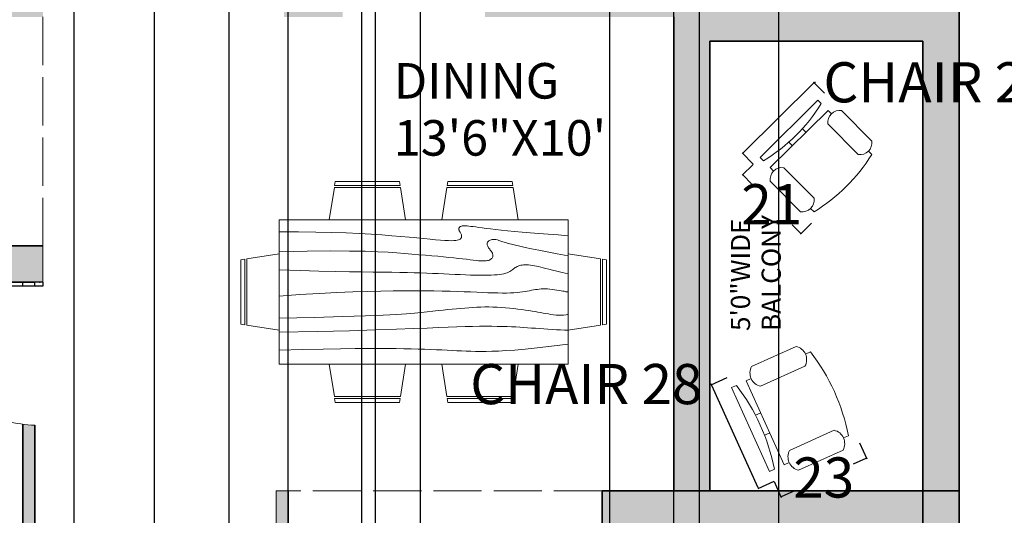
# Model space of a CAD drawing. Units: inches. Extents: x 300 to 1007, y 2 to 1069.
# Tile 10 of 12: x 617 to 862, y 743 to 867. Entities that reach past the tile are written whole.
import ezdxf

# ---------------------------------------------------------------- set-up
doc = ezdxf.new("R2010")
doc.units = ezdxf.units.IN
doc.header["$MEASUREMENT"] = 0
doc.linetypes.add('ACAD_ISO02W100', pattern=[15, 12, -3])
for name, color, linetype, lineweight in [('A-ANNO-DIMS', 2, 'Continuous', 18), ('A-AREA-IDEN', 7, 'Continuous', 18), ('A-DOOR', 3, 'Continuous', 25), ('A-DOOR-SWNG', 3, 'ACAD_ISO02W100', 13), ('A-FURN', 8, 'Continuous', 18), ('A-WALL', 7, 'Continuous', 35), ('A-WALL-OVHD', 8, 'ACAD_ISO02W100', 18)]:
    doc.layers.add(name, color=color, linetype=linetype, lineweight=lineweight)
doc.layers.add('A-WALL-PATT', color=9, linetype='Continuous', lineweight=9, true_color=0xc7c8ca)
doc.styles.get("Standard").update_dxf_attribs({"font": 'arial.ttf'})
doc.dimstyles.get("Standard").update_dxf_attribs({"dimtxt": 10, "dimasz": 0.18, "dimexe": 0.18, "dimexo": 0.0625, "dimgap": 0.09, "dimtad": 0, "dimtih": 1, "dimtoh": 1, "dimdec": 0, "dimzin": 0, "dimdsep": 46, "dimlunit": 3, "dimtxsty": 'Standard', "dimcen": 0.09, "dimadec": 0, "dimazin": 0, "dimtfac": 1, "dimtdec": 0, "dimtofl": 0, "dimtmove": 0, "dimatfit": 3, "dimfxl": 1, "dimtolj": 1, "dimtzin": 0, "dimarcsym": 0})

# ---------------------------------------------------------------- blocks, each defined once
blk = doc.blocks.new('Dining Set - 36 x 72 in.')
for p, q in [((-22, 27.5), (-22.1562, 26.50042)), ((-22, 27.5), (-6, 27.5)), ((-5.8437, 26.49966), (-6, 27.5)), ((6, 27.5), (5.8438, 26.50042)), ((6, 27.5), (22, 27.5)), ((22.1563, 26.49966), (22, 27.5)), ((-22.2343, 26.00059), (-23.4847, 17.99762)), ((-22.2304, 26), (-5.7608, 26)), ((-5.8416, 26.5), (-22.1534, 26.5)), ((-4.5152, 17.99762), (-5.7655, 25.99926)), ((5.7657, 26.00059), (4.5153, 17.99762)), ((5.7696, 26), (22.2392, 26)), ((22.1584, 26.5), (5.8466, 26.5)), ((23.4848, 17.99762), (22.2345, 25.99926)), ((36, 18), (-36, 18)), ((-36, 18), (-36, -18)), ((36, -18), (36, 18)), ((-45.5, 8), (-44.5004, 8.15617)), ((-45.5, 8), (-45.5, -8)), ((-44.5, -8.15843), (-44.5, 8.15338)), ((-44.0006, 8.23428), (-35.9976, 9.48474)), ((-44, 8.23041), (-44, -8.23915)), ((44.0006, 8.23428), (35.9976, 9.48474)), ((44, 8.23041), (44, -8.23915)), ((44.5, -8.15843), (44.5, 8.15338)), ((45.5, 8), (44.5005, 8.15617)), ((45.5, 8), (45.5, -8)), ((-44.4997, -8.15631), (-45.5, -8)), ((-35.9976, -9.48476), (-43.9993, -8.2345)), ((35.9976, -9.48476), (43.9993, -8.2345)), ((44.4997, -8.15631), (45.5, -8)), ((-36, -18), (36, -18)), ((-22.2343, -26.0006), (-23.4847, -17.99762)), ((-4.5152, -17.99762), (-5.7655, -25.99928)), ((5.7657, -26.0006), (4.5153, -17.99762)), ((23.4848, -17.99762), (22.2345, -25.99928)), ((-22.2304, -26), (-5.7608, -26)), ((-22, -27.5), (-22.1562, -26.50044)), ((-5.8416, -26.5), (-22.1534, -26.5)), ((-5.8437, -26.49967), (-6, -27.5)), ((5.7696, -26), (22.2392, -26)), ((6, -27.5), (5.8438, -26.50044)), ((22.1584, -26.5), (5.8466, -26.5)), ((22.1563, -26.49967), (22, -27.5)), ((-22, -27.5), (-6, -27.5)), ((6, -27.5), (22, -27.5))]:
    blk.add_line(p, q)
for points in [[(-36, 15), (-31.1772, 14.97754), (-26.8079, 14.91406), (-22.8538, 14.81543), (-19.276, 14.6875), (-16.0362, 14.53613), (-13.0957, 14.36718), (-10.4159, 14.18652), (-7.9583, 14), (-5.6904, 13.81315), (-3.6035, 13.63021), (-1.6954, 13.45508), (0.0365, 13.29166), (1.5945, 13.14388), (2.9811, 13.01562), (4.1988, 12.9108), (5.25, 12.83333), (6.1393, 12.78613), (6.8802, 12.76823), (7.4883, 12.77767), (7.9792, 12.8125), (8.3685, 12.87077), (8.6719, 12.95052), (8.9049, 13.0498), (9.0833, 13.16666), (9.2205, 13.29899), (9.3216, 13.44401), (9.3895, 13.59879), (9.4271, 13.76041), (9.4373, 13.92594), (9.4232, 14.09245), (9.3875, 14.257), (9.3333, 14.41666), (9.2638, 14.56917), (9.1836, 14.71484), (9.0975, 14.85465), (9.0104, 14.98958), (8.9272, 15.1206), (8.8529, 15.2487), (8.7922, 15.37483), (8.75, 15.5), (8.7305, 15.62467), (8.7344, 15.74739), (8.7617, 15.86621), (8.8125, 15.97916), (8.8867, 16.08431), (8.9844, 16.17968), (9.1055, 16.26334), (9.25, 16.33333), (9.4189, 16.38802), (9.6172, 16.42708), (9.8506, 16.45052), (10.125, 16.45833), (10.4463, 16.45052), (10.8203, 16.42708), (11.2529, 16.38802), (11.75, 16.33333), (12.3184, 16.26318), (12.9694, 16.17838), (13.7151, 16.07991), (14.5677, 15.96875), (15.5395, 15.84586), (16.6426, 15.71224), (17.8893, 15.56884), (19.2917, 15.41666), (20.859, 15.25667), (22.5879, 15.08984), (24.4721, 14.91715), (26.5052, 14.73958), (28.6809, 14.5581), (30.9929, 14.3737), (33.4347, 14.18733), (36, 14)], [(-36, 10), (-28.9766, 10.14274), (-23.1725, 10.20442), (-18.4241, 10.19775), (-14.5677, 10.13541), (-11.4399, 10.03011), (-8.877, 9.89453), (-6.7154, 9.74137), (-4.7917, 9.58333), (-2.9698, 9.43082), (-1.2246, 9.28515), (0.4415, 9.14534), (2.026, 9.01041), (3.5266, 8.87939), (4.9408, 8.7513), (6.266, 8.62516), (7.5, 8.5), (8.6411, 8.37549), (9.6914, 8.2539), (10.6538, 8.13818), (11.5312, 8.03125), (12.3267, 7.93603), (13.043, 7.85547), (13.6831, 7.79248), (14.25, 7.75), (14.7471, 7.7303), (15.1797, 7.73307), (15.5537, 7.75732), (15.875, 7.80208), (16.1494, 7.86637), (16.3828, 7.94922), (16.5811, 8.04964), (16.75, 8.16666), (16.8944, 8.29915), (17.0143, 8.44531), (17.1089, 8.60319), (17.1771, 8.77083), (17.218, 8.94629), (17.2305, 9.1276), (17.2137, 9.31282), (17.1667, 9.5), (17.0895, 9.6875), (16.987, 9.875), (16.8649, 10.0625), (16.7292, 10.25), (16.5856, 10.4375), (16.4401, 10.625), (16.2985, 10.8125), (16.1667, 11), (16.05, 11.18733), (15.9518, 11.3737), (15.8752, 11.5581), (15.8229, 11.73958), (15.798, 11.91715), (15.8034, 12.08984), (15.842, 12.25667), (15.9167, 12.41666), (16.0295, 12.56836), (16.1784, 12.70833), (16.3605, 12.83268), (16.5729, 12.9375), (16.8127, 13.01888), (17.0768, 13.07291), (17.3625, 13.0957), (17.6667, 13.08333), (17.9894, 13.03312), (18.3418, 12.94726), (18.7382, 12.82918), (19.1927, 12.68229), (19.7195, 12.51001), (20.3327, 12.31575), (21.0465, 12.10294), (21.875, 11.875), (22.8357, 11.63354), (23.959, 11.37304), (25.2786, 11.08618), (26.8282, 10.76562), (28.6414, 10.40405), (30.752, 9.99414), (33.1936, 9.52856), (36, 9)], [(-36, 5.5), (-30.7157, 5.3348), (-26.069, 5.20963), (-21.9946, 5.11767), (-18.4271, 5.05208), (-15.3009, 5.00602), (-12.5508, 4.97265), (-10.1112, 4.94515), (-7.9167, 4.91666), (-5.909, 4.88167), (-4.0586, 4.83984), (-2.3429, 4.79215), (-0.7396, 4.73958), (0.7739, 4.6831), (2.22, 4.6237), (3.6213, 4.56233), (5, 4.5), (6.373, 4.43782), (7.7344, 4.3776), (9.0723, 4.32129), (10.375, 4.27083), (11.6309, 4.22819), (12.8281, 4.19531), (13.9551, 4.17415), (15, 4.16666), (15.954, 4.17448), (16.819, 4.19791), (17.6001, 4.23698), (18.3021, 4.29166), (18.9299, 4.36198), (19.4883, 4.44791), (19.9823, 4.54948), (20.4167, 4.66666), (20.7969, 4.79899), (21.1302, 4.94401), (21.4245, 5.09879), (21.6875, 5.26041), (21.9271, 5.42594), (22.1511, 5.59245), (22.3672, 5.757), (22.5834, 5.91666), (22.8065, 6.06868), (23.0404, 6.21093), (23.2879, 6.34147), (23.5521, 6.45833), (23.8358, 6.55957), (24.142, 6.64323), (24.4735, 6.70735), (24.8334, 6.75), (25.2235, 6.76969), (25.642, 6.76692), (26.0858, 6.74267), (26.5521, 6.69791), (27.0379, 6.63362), (27.5404, 6.55078), (28.0565, 6.45036), (28.5834, 6.33333), (29.1242, 6.19987), (29.7071, 6.04687), (30.3661, 5.87044), (31.1354, 5.66666), (32.0493, 5.43164), (33.142, 5.16146), (34.4475, 4.85221), (36, 4.5)], [(-36, -1), (-30.7915, -0.6591), (-26.0195, -0.38216), (-21.6519, -0.16284), (-17.6563, 0.00521), (-14.0005, 0.12833), (-10.6523, 0.21289), (-7.5796, 0.26522), (-4.75, 0.29166), (-2.134, 0.29793), (0.2878, 0.28711), (2.5317, 0.26163), (4.6146, 0.22396), (6.5529, 0.17651), (8.3633, 0.12174), (10.0623, 0.06209), (11.6667, 0), (13.1899, -0.06201), (14.6341, -0.1211), (15.9982, -0.17432), (17.2813, -0.21875), (18.4823, -0.25147), (19.6003, -0.26953), (20.6343, -0.27002), (21.5834, -0.25), (22.4481, -0.20768), (23.2357, -0.14584), (23.9549, -0.06836), (24.6146, 0.02083), (25.2235, 0.11784), (25.7904, 0.21875), (26.3241, 0.31966), (26.8334, 0.41666), (27.3265, 0.50618), (27.8099, 0.58593), (28.2894, 0.65397), (28.7709, 0.70833), (29.2601, 0.74707), (29.763, 0.76823), (30.2855, 0.76985), (30.8334, 0.75), (31.4088, 0.70784), (31.9994, 0.64713), (32.589, 0.57275), (33.1615, 0.48958), (33.7008, 0.4025), (34.1908, 0.3164), (34.6153, 0.23616), (34.9584, 0.16666), (35.2099, 0.11165), (35.3848, 0.07031), (35.504, 0.04069), (35.5886, 0.02083), (35.6594, 0.00879), (35.7377, 0.0026), (35.8442, 0.00032), (36, 0)], [(-36, -6.5), (-27.1843, -6.31267), (-20.084, -6.1263), (-14.469, -5.9419), (-10.1094, -5.76042), (-6.7752, -5.58285), (-4.2363, -5.41016), (-2.2629, -5.24333), (-0.625, -5.08334), (0.8708, -4.93099), (2.2715, -4.78646), (3.5872, -4.64974), (4.8281, -4.52084), (6.0046, -4.39974), (7.127, -4.28646), (8.2053, -4.18099), (9.25, -4.08334), (10.2705, -3.99382), (11.2734, -3.91407), (12.2647, -3.84603), (13.25, -3.79167), (14.2354, -3.75293), (15.2266, -3.73177), (16.2295, -3.73015), (17.25, -3.75), (18.2912, -3.79248), (19.3451, -3.85547), (20.4009, -3.93604), (21.4479, -4.03125), (22.4754, -4.13819), (23.4727, -4.25391), (24.4289, -4.37549), (25.3334, -4.5), (26.1785, -4.62492), (26.9694, -4.74935), (27.7145, -4.87281), (28.4219, -4.99479), (29.1, -5.11483), (29.7572, -5.23242), (30.4016, -5.34709), (31.0417, -5.45834), (31.6837, -5.56437), (32.3262, -5.65821), (32.9658, -5.73153), (33.599, -5.77604), (34.2224, -5.78345), (34.8327, -5.74545), (35.4264, -5.65373), (36, -5.5)], [(-36, -10), (-26.4022, -9.81299), (-18.4675, -9.62891), (-11.9839, -9.45069), (-6.7396, -9.28125), (-2.5226, -9.12354), (0.8789, -8.98047), (3.6769, -8.85498), (6.0833, -8.75), (8.2767, -8.66765), (10.3021, -8.60677), (12.1712, -8.56543), (13.8958, -8.54167), (15.4876, -8.53353), (16.9583, -8.53907), (18.3197, -8.55632), (19.5834, -8.58334), (20.7616, -8.61841), (21.8685, -8.66081), (22.9188, -8.71004), (23.9271, -8.76563), (24.9081, -8.82707), (25.8763, -8.89388), (26.8465, -8.96558), (27.8334, -9.04167), (28.8474, -9.12118), (29.8828, -9.20117), (30.93, -9.27824), (31.9792, -9.34896), (33.0205, -9.40991), (34.0443, -9.45768), (35.0407, -9.48885), (36, -9.5)], [(-36, -14.5), (-30.0881, -14.33513), (-25.0332, -14.21224), (-20.7312, -14.12647), (-17.0781, -14.07292), (-13.97, -14.04671), (-11.3027, -14.04297), (-8.9724, -14.05681), (-6.875, -14.08334), (-4.9224, -14.11833), (-3.0905, -14.16016), (-1.3709, -14.20785), (0.2448, -14.26042), (1.7647, -14.3169), (3.1973, -14.3763), (4.5507, -14.43767), (5.8333, -14.5), (7.0554, -14.5621), (8.235, -14.62175), (9.3922, -14.67652), (10.5469, -14.72396), (11.7192, -14.76164), (12.929, -14.78711), (14.1965, -14.79794), (15.5417, -14.79167), (16.9933, -14.76424), (18.6152, -14.70508), (20.4804, -14.60197), (22.6615, -14.44271), (25.2312, -14.21509), (28.2624, -13.9069), (31.8277, -13.50594), (36, -13)]]:
    blk.add_lwpolyline(points)
blk = doc.blocks.new('Chair - Desk')
for p, q in [((-8.5, 0), (-8.5, -1)), ((-8.5, 0), (8.5, 0)), ((8.5, 0), (8.5, -1)), ((-8.5, -3), (-8.5, -4)), ((-8.5, -3), (8.5, -3)), ((-2, -3), (-2, -1.9355)), ((2, -1.9576), (2, -3)), ((8.5, -3), (8.5, -4)), ((-10.5, -5), (-10.5, -14)), ((-6.5, -14), (-6.5, -5)), ((6.5, -5), (6.5, -14)), ((10.5, -14), (10.5, -5)), ((-8.5, -15), (-8.5, -16)), ((8.5, -15), (8.5, -16))]:
    blk.add_line(p, q)
for centre, radius, start, end in [((0, 34.625), 36.625, 256.5803, 283.4197), ((-8.5, -6.5), 2.5, 36.8699, 143.1301), ((8.5, -6.5), 2.5, 36.8699, 143.1301), ((-8.5, -12.5), 2.5, 216.8699, 323.1301), ((8.5, -12.5), 2.5, 216.8699, 323.1301), ((0, 19.625), 36.625, 256.5803, 283.4197)]:
    blk.add_arc(centre, radius, start, end)
blk = doc.blocks.new('*D23')
at = {"layer": 'A-ANNO-DIMS', "color": 0, "lineweight": -2, "transparency": 16777216}
for p, q in [((797.11, 833.59), (814.61, 850.93)), ((817.34, 848.44), (814.61, 851.18)), ((814.74, 851.06), (814.87, 851.18)), ((814.87, 851.18), (815.05, 851.18)), ((799.58, 830.84), (796.86, 833.59))]:
    blk.add_line(p, q, dxfattribs=at)
at = {"layer": 'A-ANNO-DIMS', "color": 0, "transparency": 16777216}
for points in [[(814.59, 850.95), (814.63, 850.91), (814.74, 851.06)], [(797.09, 833.61), (797.13, 833.57), (796.98, 833.46)]]:
    blk.add_solid(points, dxfattribs=at)
at = {"layer": 'Defpoints', "color": 0, "transparency": 16777216}
for p in [(814.74, 851.06), (817.38, 848.39), (799.62, 830.8)]:
    blk.add_point(p, dxfattribs=at)
at = {"layer": 'A-ANNO-DIMS', "color": 0, "transparency": 16777216, "insert": (845.95, 851.18), "char_height": 10, "attachment_point": 5}
blk.add_mtext('\\A1;CHAIR 25', dxfattribs=at)
blk = doc.blocks.new('*D24')
at = {"layer": 'A-ANNO-DIMS', "color": 0, "lineweight": -2, "transparency": 16777216}
for p, q in [((799.58, 830.76), (796.83, 828.04)), ((797.08, 828.03), (799.16, 825.94)), ((814.1, 816.1), (811.35, 813.38)), ((811.35, 813.63), (809.28, 815.72))]:
    blk.add_line(p, q, dxfattribs=at)
at = {"layer": 'A-ANNO-DIMS', "color": 0, "transparency": 16777216}
for points in [[(797.11, 828.05), (797.06, 828.01), (796.96, 828.16)], [(811.37, 813.65), (811.33, 813.61), (811.48, 813.5)]]:
    blk.add_solid(points, dxfattribs=at)
at = {"layer": 'Defpoints', "color": 0, "transparency": 16777216}
for p in [(799.62, 830.8), (796.96, 828.16), (814.14, 816.14)]:
    blk.add_point(p, dxfattribs=at)
at = {"layer": 'A-ANNO-DIMS', "color": 0, "transparency": 16777216, "insert": (804.22, 820.83), "char_height": 10, "attachment_point": 5}
blk.add_mtext('\\A1;21', dxfattribs=at)
blk = doc.blocks.new('*D25')
at = {"layer": 'A-ANNO-DIMS', "color": 0, "lineweight": -2, "transparency": 16777216}
for p, q in [((792.99, 777.62), (789.02, 775.82)), ((789.11, 776.06), (788.93, 776.06)), ((789.18, 775.89), (789.11, 776.06)), ((800.8, 750.26), (789.26, 775.73)), ((804.68, 751.83), (800.71, 750.02))]:
    blk.add_line(p, q, dxfattribs=at)
at = {"layer": 'A-ANNO-DIMS', "color": 0, "transparency": 16777216}
for points in [[(789.28, 775.74), (789.23, 775.71), (789.18, 775.89)], [(800.83, 750.27), (800.77, 750.25), (800.87, 750.1)]]:
    blk.add_solid(points, dxfattribs=at)
at = {"layer": 'Defpoints', "color": 0, "transparency": 16777216}
for p in [(793.05, 777.64), (789.18, 775.89), (804.74, 751.85)]:
    blk.add_point(p, dxfattribs=at)
at = {"layer": 'A-ANNO-DIMS', "color": 0, "transparency": 16777216, "insert": (758.05, 776.06), "char_height": 10, "attachment_point": 5}
blk.add_mtext('\\A1;CHAIR 28', dxfattribs=at)
blk = doc.blocks.new('*D26')
at = {"layer": 'A-ANNO-DIMS', "color": 0, "lineweight": -2, "transparency": 16777216}
for p, q in [((826.06, 761.44), (827.86, 757.47)), ((827.62, 757.56), (824.48, 756.13)), ((804.77, 751.79), (806.57, 747.82)), ((806.66, 748.06), (809.8, 749.48))]:
    blk.add_line(p, q, dxfattribs=at)
at = {"layer": 'A-ANNO-DIMS', "color": 0, "transparency": 16777216}
for points in [[(827.61, 757.59), (827.63, 757.53), (827.78, 757.63)], [(806.65, 748.08), (806.67, 748.03), (806.5, 747.98)]]:
    blk.add_solid(points, dxfattribs=at)
at = {"layer": 'Defpoints', "color": 0, "transparency": 16777216}
for p in [(826.03, 761.5), (804.74, 751.85), (806.5, 747.98)]:
    blk.add_point(p, dxfattribs=at)
at = {"layer": 'A-ANNO-DIMS', "color": 0, "transparency": 16777216, "insert": (817.14, 752.81), "char_height": 10, "attachment_point": 5}
blk.add_mtext('\\A1;23', dxfattribs=at)
blk = doc.blocks.new('*D78')
at = {"layer": 'A-ANNO-DIMS', "color": 0, "lineweight": -2, "transparency": 16777216}
for p, q in [((850.89, 999.45), (974.48, 999.45)), ((974.3, 999.27), (974.3, 809.65)), ((974.3, 609.63), (974.3, 799.25)), ((841.89, 609.45), (974.48, 609.45))]:
    blk.add_line(p, q, dxfattribs=at)
at = {"layer": 'A-ANNO-DIMS', "color": 0, "transparency": 16777216}
for points in [[(974.27, 999.27), (974.33, 999.27), (974.3, 999.45)], [(974.27, 609.63), (974.33, 609.63), (974.3, 609.45)]]:
    blk.add_solid(points, dxfattribs=at)
at = {"layer": 'Defpoints', "color": 0, "transparency": 16777216}
for p in [(850.83, 999.45), (974.3, 999.45), (841.83, 609.45)]:
    blk.add_point(p, dxfattribs=at)
at = {"layer": 'A-ANNO-DIMS', "color": 0, "transparency": 16777216, "insert": (974.3, 804.45), "char_height": 10, "attachment_point": 5}
blk.add_mtext('\\A1;390', dxfattribs=at)
blk = doc.blocks.new('*D80')
at = {"layer": 'A-ANNO-DIMS', "color": 0, "lineweight": -2, "transparency": 16777216}
for p, q in [((683.83, 717.31), (683.83, 1063.03)), ((684.01, 1062.85), (705.41, 1062.85)), ((705.59, 717.31), (705.59, 1063.03)), ((705.59, 1062.85), (705.77, 1062.85))]:
    blk.add_line(p, q, dxfattribs=at)
at = {"layer": 'A-ANNO-DIMS', "color": 0, "transparency": 16777216}
for points in [[(684.01, 1062.88), (684.01, 1062.82), (683.83, 1062.85)], [(705.41, 1062.88), (705.41, 1062.82), (705.59, 1062.85)]]:
    blk.add_solid(points, dxfattribs=at)
at = {"layer": 'Defpoints', "color": 0, "transparency": 16777216}
for p in [(705.59, 1062.85), (683.83, 717.25), (705.59, 717.25)]:
    blk.add_point(p, dxfattribs=at)
at = {"layer": 'A-ANNO-DIMS', "color": 0, "transparency": 16777216, "insert": (726.71, 1062.85), "char_height": 10, "attachment_point": 5}
blk.add_mtext('\\A1;21.767', dxfattribs=at)
blk = doc.blocks.new('*D82')
at = {"layer": 'A-ANNO-DIMS', "color": 0, "lineweight": -2, "transparency": 16777216}
for p, q in [((763.9, 700.01), (763.9, 1063.03)), ((764.08, 1062.85), (779.65, 1062.85)), ((779.83, 700.01), (779.83, 1063.03)), ((779.83, 1062.85), (780.01, 1062.85))]:
    blk.add_line(p, q, dxfattribs=at)
at = {"layer": 'A-ANNO-DIMS', "color": 0, "transparency": 16777216}
for points in [[(764.08, 1062.88), (764.08, 1062.82), (763.9, 1062.85)], [(779.65, 1062.88), (779.65, 1062.82), (779.83, 1062.85)]]:
    blk.add_solid(points, dxfattribs=at)
at = {"layer": 'Defpoints', "color": 0, "transparency": 16777216}
for p in [(779.83, 1062.85), (763.9, 699.95), (779.83, 699.95)]:
    blk.add_point(p, dxfattribs=at)
at = {"layer": 'A-ANNO-DIMS', "color": 0, "transparency": 16777216, "insert": (800.38, 1062.85), "char_height": 10, "attachment_point": 5}
blk.add_mtext('\\A1;15.927', dxfattribs=at)
blk = doc.blocks.new('*D86')
at = {"layer": 'A-ANNO-DIMS', "color": 0, "lineweight": -2, "transparency": 16777216}
for p, q in [((805.95, 235.15), (805.95, 1063.03)), ((806.13, 1062.85), (822.02, 1062.85)), ((864.07, 1062.85), (848.18, 1062.85)), ((864.25, 235.15), (864.25, 1063.03))]:
    blk.add_line(p, q, dxfattribs=at)
at = {"layer": 'A-ANNO-DIMS', "color": 0, "transparency": 16777216}
for points in [[(806.13, 1062.88), (806.13, 1062.82), (805.95, 1062.85)], [(864.07, 1062.88), (864.07, 1062.82), (864.25, 1062.85)]]:
    blk.add_solid(points, dxfattribs=at)
at = {"layer": 'Defpoints', "color": 0, "transparency": 16777216}
for p in [(864.25, 1062.85), (805.95, 235.08), (864.25, 235.08)]:
    blk.add_point(p, dxfattribs=at)
at = {"layer": 'A-ANNO-DIMS', "color": 0, "transparency": 16777216, "insert": (835.1, 1062.85), "char_height": 10, "attachment_point": 5}
blk.add_mtext('\\A1;58.3', dxfattribs=at)
blk = doc.blocks.new('*D99')
at = {"layer": 'A-ANNO-DIMS', "color": 0, "lineweight": -2, "transparency": 16777216}
for p, q in [((604.49, 482.45), (604.49, 1063.03)), ((604.67, 1062.85), (619.83, 1062.85)), ((668.97, 1062.85), (653.8, 1062.85)), ((669.15, 482.45), (669.15, 1063.03))]:
    blk.add_line(p, q, dxfattribs=at)
at = {"layer": 'A-ANNO-DIMS', "color": 0, "transparency": 16777216}
for points in [[(604.67, 1062.88), (604.67, 1062.82), (604.49, 1062.85)], [(668.97, 1062.88), (668.97, 1062.82), (669.15, 1062.85)]]:
    blk.add_solid(points, dxfattribs=at)
at = {"layer": 'Defpoints', "color": 0, "transparency": 16777216}
for p in [(669.15, 1062.85), (604.49, 482.38), (669.15, 482.38)]:
    blk.add_point(p, dxfattribs=at)
at = {"layer": 'A-ANNO-DIMS', "color": 0, "transparency": 16777216, "insert": (636.82, 1062.85), "char_height": 10, "attachment_point": 5}
blk.add_mtext('\\A1;64.66', dxfattribs=at)
blk = doc.blocks.new('*D100')
at = {"layer": 'A-ANNO-DIMS', "color": 0, "lineweight": -2, "transparency": 16777216}
for p, q in [((716.78, 482.45), (716.78, 1063.03)), ((716.96, 1062.85), (734.53, 1062.85)), ((786.04, 1062.85), (768.47, 1062.85)), ((786.22, 482.45), (786.22, 1063.03))]:
    blk.add_line(p, q, dxfattribs=at)
at = {"layer": 'A-ANNO-DIMS', "color": 0, "transparency": 16777216}
for points in [[(716.96, 1062.88), (716.96, 1062.82), (716.78, 1062.85)], [(786.04, 1062.88), (786.04, 1062.82), (786.22, 1062.85)]]:
    blk.add_solid(points, dxfattribs=at)
at = {"layer": 'Defpoints', "color": 0, "transparency": 16777216}
for p in [(786.22, 1062.85), (716.78, 482.38), (786.22, 482.38)]:
    blk.add_point(p, dxfattribs=at)
at = {"layer": 'A-ANNO-DIMS', "color": 0, "transparency": 16777216, "insert": (751.5, 1062.85), "char_height": 10, "attachment_point": 5}
blk.add_mtext('\\A1;69.44', dxfattribs=at)
blk = doc.blocks.new('*D106')
at = {"layer": 'A-ANNO-DIMS', "color": 0, "lineweight": -2, "transparency": 16777216}
for p, q in [((582.11, 990.38), (582.11, 8.45)), ((630.49, 990.38), (630.49, 8.45)), ((582.29, 8.63), (589.12, 8.63)), ((630.31, 8.63), (623.47, 8.63))]:
    blk.add_line(p, q, dxfattribs=at)
at = {"layer": 'A-ANNO-DIMS', "color": 0, "transparency": 16777216}
for points in [[(582.29, 8.66), (582.29, 8.6), (582.11, 8.63)], [(630.31, 8.66), (630.31, 8.6), (630.49, 8.63)]]:
    blk.add_solid(points, dxfattribs=at)
at = {"layer": 'Defpoints', "color": 0, "transparency": 16777216}
for p in [(582.11, 990.45), (630.49, 990.45), (630.49, 8.63)]:
    blk.add_point(p, dxfattribs=at)
at = {"layer": 'A-ANNO-DIMS', "color": 0, "transparency": 16777216, "insert": (606.3, 8.63), "char_height": 10, "attachment_point": 5}
blk.add_mtext('\\A1;48.38', dxfattribs=at)
blk = doc.blocks.new('*D107')
at = {"layer": 'A-ANNO-DIMS', "color": 0, "lineweight": -2, "transparency": 16777216}
for p, q in [((630.49, 990.38), (630.49, 8.45)), ((650.47, 990.38), (650.47, 8.45)), ((630.67, 8.63), (650.29, 8.63)), ((650.47, 8.63), (650.65, 8.63))]:
    blk.add_line(p, q, dxfattribs=at)
at = {"layer": 'A-ANNO-DIMS', "color": 0, "transparency": 16777216}
for points in [[(630.67, 8.66), (630.67, 8.6), (630.49, 8.63)], [(650.29, 8.66), (650.29, 8.6), (650.47, 8.63)]]:
    blk.add_solid(points, dxfattribs=at)
at = {"layer": 'Defpoints', "color": 0, "transparency": 16777216}
for p in [(630.49, 990.45), (650.47, 990.45), (650.47, 8.63)]:
    blk.add_point(p, dxfattribs=at)
at = {"layer": 'A-ANNO-DIMS', "color": 0, "transparency": 16777216, "insert": (667.15, 8.63), "char_height": 10, "attachment_point": 5}
blk.add_mtext('\\A1;19.98', dxfattribs=at)
blk = doc.blocks.new('*D108')
at = {"layer": 'A-ANNO-DIMS', "color": 0, "lineweight": -2, "transparency": 16777216}
for p, q in [((650.47, 990.38), (650.47, 8.45)), ((702.09, 990.38), (702.09, 8.45)), ((650.65, 8.63), (659.37, 8.63)), ((701.91, 8.63), (693.19, 8.63))]:
    blk.add_line(p, q, dxfattribs=at)
at = {"layer": 'A-ANNO-DIMS', "color": 0, "transparency": 16777216}
for points in [[(650.65, 8.66), (650.65, 8.6), (650.47, 8.63)], [(701.91, 8.66), (701.91, 8.6), (702.09, 8.63)]]:
    blk.add_solid(points, dxfattribs=at)
at = {"layer": 'Defpoints', "color": 0, "transparency": 16777216}
for p in [(650.47, 990.45), (702.09, 990.45), (702.09, 8.63)]:
    blk.add_point(p, dxfattribs=at)
at = {"layer": 'A-ANNO-DIMS', "color": 0, "transparency": 16777216, "insert": (676.28, 8.63), "char_height": 10, "attachment_point": 5}
blk.add_mtext('\\A1;51.62', dxfattribs=at)
blk = doc.blocks.new('*D113')
at = {"layer": 'A-ANNO-DIMS', "color": 0, "lineweight": -2, "transparency": 16777216}
for p, q in [((621.98, 801.45), (622.16, 801.45)), ((622.07, 801.36), (622.07, 801.54)), ((581.05, 761.83), (596.3, 776.56)), ((580.87, 761.83), (581.05, 761.83))]:
    blk.add_line(p, q, dxfattribs=at)
at = {"layer": 'A-ANNO-DIMS', "color": 0, "transparency": 16777216}
blk.add_solid([(596.28, 776.58), (596.32, 776.54), (596.43, 776.68)], dxfattribs=at)
at = {"layer": 'Defpoints', "color": 0, "transparency": 16777216}
for p in [(622.07, 801.45), (596.43, 776.68)]:
    blk.add_point(p, dxfattribs=at)
at = {"layer": 'A-ANNO-DIMS', "color": 0, "transparency": 16777216, "insert": (555.25, 761.83), "char_height": 10, "attachment_point": 5}
blk.add_mtext('\\A1;R35.644', dxfattribs=at)

msp = doc.modelspace()

# ---------------------------------------------------------------- hatches: boundary and pattern name
at = {"layer": 'A-WALL-PATT'}
h = msp.add_hatch(color=256, dxfattribs=at)
h.dxf.hatch_style = 1
h.paths.add_polyline_path([(546.104, 999.4468), (478.8267, 999.4468), (478.8267, 869.2798, -0.06322715), (487.8267, 868.1328), (487.8267, 990.4468), (546.104, 990.4468)])
h.paths.add_polyline_path([(630.4852, 999.4468), (582.106, 999.4468), (582.106, 990.4468), (613.8267, 990.4468), (613.8267, 867.4468), (622.8267, 867.4468), (622.8267, 990.4468), (630.4852, 990.4468)])
h.paths.add_polyline_path([(702.0883, 999.4468), (650.4653, 999.4468), (650.4653, 990.4468), (682.8267, 990.4468), (682.8267, 960.0824, -0.02530575), (685.8267, 960.0478), (685.8267, 990.4468), (702.0883, 990.4468)])
h.paths.add_polyline_path([(850.8267, 999.4468), (737.5888, 999.4468), (737.5888, 990.4468), (841.8267, 990.4468), (841.8267, 950.5685), (850.8267, 950.5685)])
h.paths.add_polyline_path([(685.8267, 930.4465), (682.8267, 930.4465), (682.8267, 888.4468), (682.8267, 867.4468), (685.8267, 867.4468), (697.4169, 867.4468), (697.4169, 870.4468), (685.8267, 870.4468), (685.8267, 888.4468)])
h.paths.add_polyline_path([(682.8267, 931.4465), (654.3436, 931.4465, 0.00843109), (654.3267, 930.4465), (682.8267, 930.4465)])
h.paths.add_polyline_path([(685.8267, 931.4465), (682.8267, 931.4465), (682.8267, 930.4465), (685.8267, 930.4465)])
h.paths.add_polyline_path([(682.8267, 888.4468), (622.8267, 888.4468), (622.8267, 885.4468), (682.8267, 885.4468)])
h.paths.add_polyline_path([(850.8267, 870.4468), (850.8267, 914.7851), (841.8267, 914.7851), (841.8267, 870.4468), (732.7101, 870.4468, -0.02120595), (732.8267, 867.4468), (779.8267, 867.4468), (779.8267, 749.4468), (782.8267, 749.4468), (788.8267, 749.4468), (788.8267, 861.4468), (841.8267, 861.4468), (841.8267, 749.4468), (850.8267, 749.4468)])
h.paths.add_polyline_path([(622.8267, 810.4468), (487.8267, 810.4468), (487.8267, 833.2626), (478.8267, 833.2626), (478.8267, 609.4468), (478.8267, 482.3847), (487.8267, 482.3847), (487.8267, 801.4468), (620.8267, 801.4468), (622.8267, 801.4468)])
h.paths.add_polyline_path([(680.8267, 729.4468), (620.8267, 729.4468), (620.8267, 765.8246, -0.02111352), (617.8267, 766.0562), (617.8267, 698.7303), (620.8267, 698.7303), (620.8267, 726.4468), (680.8267, 726.4468)])
h.paths.add_polyline_path([(620.8267, 668.8122, -0.02498293), (617.8267, 668.6448), (617.8267, 618.4468), (600.3357, 618.4468), (600.3357, 609.4468), (652.9929, 609.4468), (652.9929, 618.4468), (620.8267, 618.4468)])
h.paths.add_polyline_path([(552.3393, 618.4468), (487.8267, 618.4468), (487.8267, 609.4468), (552.3393, 609.4468)], flags=17)
h.paths.add_polyline_path([(694.5763, 618.4468), (683.8267, 618.4468), (683.8267, 726.4468), (683.8267, 749.4468), (680.8267, 749.4468), (680.8267, 740.4468), (680.8267, 726.4468), (680.8267, 618.4468), (674.1573, 618.4468), (674.1573, 609.4468), (680.8267, 609.4468), (694.5763, 609.4468)])
h.paths.add_polyline_path([(850.8267, 642.8902), (841.8267, 642.8902), (841.8267, 618.4468), (782.8267, 618.4468), (782.8267, 708.0513, -0.02308839), (779.8267, 707.9092), (779.8267, 618.4468), (730.1068, 618.4468), (730.1068, 609.4468), (779.8267, 609.4468), (841.8267, 609.4468), (841.8267, 482.3847), (850.8267, 482.3847)])
h.paths.add_polyline_path([(850.8267, 749.4468), (841.8267, 749.4468), (841.8267, 705.9119), (850.8267, 705.9119)])
h.paths.add_polyline_path([(841.8267, 749.4468), (782.8267, 749.4468), (779.8267, 749.4468), (761.9959, 749.4468), (761.9959, 740.4468), (779.8267, 740.4468), (812.3267, 740.4468), (841.8267, 740.4468)])
h.paths.add_polyline_path([(669.1457, 482.3847), (604.489, 482.3847), (604.489, 473.3847), (631.1217, 473.3847), (631.1217, 436.0244, -0.02504709), (634.1217, 436.1748), (634.1217, 436.4367), (634.1217, 473.3847), (669.1457, 473.3847)], flags=17)
h.paths.add_polyline_path([(580.5305, 482.3847), (571.1217, 482.3847), (541.0813, 482.3847), (541.0813, 473.3847), (562.1217, 473.3847), (562.1217, 326.3847), (571.1217, 326.3847), (571.1217, 362.3847), (631.1217, 362.3847), (631.1217, 326.3847), (706.9024, 326.3847, -0.02105388), (706.9999, 329.3847), (634.1217, 329.3847), (634.1217, 365.3847), (634.1217, 406.1748), (631.1217, 406.1748), (631.1217, 365.3847), (571.1217, 365.3847), (571.1217, 473.3847), (580.5305, 473.3847)])
h.paths.add_polyline_path([(493.4756, 482.3847), (420.1217, 482.3847), (420.1217, 445.3134), (429.1217, 445.3134), (429.1217, 473.3847), (493.4756, 473.3847)])
h.paths.add_polyline_path([(786.2236, 482.3847), (716.7793, 482.3847), (716.7793, 473.3847), (766.1217, 473.3847), (766.1217, 329.3847), (742.5583, 329.3847), (742.5583, 326.3847), (766.1217, 326.3847), (766.1217, 316.0647), (769.1217, 316.0647), (769.1217, 326.3847), (769.1217, 473.3847), (786.2236, 473.3847)])
h.paths.add_polyline_path([(910.1217, 482.3847), (822.7166, 482.3847), (822.7166, 473.3847), (901.1217, 473.3847), (901.1217, 402.5393), (910.1217, 402.5393)])
h.paths.add_polyline_path([(910.1217, 366.1034), (901.1217, 366.1034), (901.1217, 329.3847), (814.1217, 329.3847), (814.1217, 312.5176), (817.1217, 312.5176), (817.1217, 326.3847), (901.1217, 326.3847), (901.1217, 293.0319), (910.1217, 293.0319), (910.1217, 326.3847)])
h.paths.add_polyline_path([(910.1217, 268.9355), (901.1217, 268.9355), (901.1217, 254.3847), (817.1217, 254.3847), (817.1217, 290.5411, -0.03396715), (814.1217, 290.3847), (814.1217, 254.3847), (775.1217, 254.3847), (775.1217, 281.5164), (769.1217, 281.5164), (769.1217, 292.1577), (766.1217, 292.1577), (766.1217, 254.3847), (766.1217, 220.1938), (775.5079, 220.1938), (775.5079, 251.3847), (817.1217, 251.3847), (901.1217, 251.3847), (901.1217, 152.3847), (819.0246, 152.3847, -0.02493798), (818.9117, 149.3847), (901.1217, 149.3847), (901.1217, 92.3847), (901.1217, 83.3847), (874.3528, 83.3847), (874.3528, 74.3847), (910.1217, 74.3847), (910.1217, 92.3847), (910.1217, 149.3847)])
h.paths.add_polyline_path([(429.1217, 325.0924), (420.1217, 325.0924), (420.1217, 263.3847), (420.1217, 244.9834), (429.1217, 244.9834), (429.1217, 269.3847), (571.1217, 269.3847), (571.1217, 272.3847), (562.1217, 272.3847), (429.1217, 272.3847)])
h.paths.add_polyline_path([(429.1217, 208.998), (420.1217, 208.998), (420.1217, 74.3847), (496.7704, 74.3847), (496.7704, 83.3847), (429.1217, 83.3847)])
h.paths.add_polyline_path([(598.4322, 83.3847), (571.1217, 83.3847), (571.1217, 122.1171), (562.1217, 122.1171), (562.1217, 83.3847), (544.6031, 83.3847), (544.6031, 74.3847), (598.4322, 74.3847)])
h.paths.add_polyline_path([(797.0822, 83.3847), (769.1217, 83.3847), (769.1217, 149.3847), (788.9123, 149.3847), (788.9123, 152.3847), (769.1217, 152.3847), (769.1217, 178.0167), (766.1217, 178.0167), (766.1217, 152.3847), (735.3598, 152.3847), (735.3598, 143.3847), (766.1217, 143.3847), (766.1217, 83.3847), (634.1217, 83.3847), (634.1217, 143.3847), (659.7326, 143.3847), (659.7326, 152.3847), (634.1217, 152.3847), (634.1217, 194.3847), (571.1217, 194.3847), (571.1217, 233.7289, -0.06379947), (562.1217, 234.7942), (562.1217, 163.4485), (567.7403, 163.4485), (567.7403, 152.3847), (571.1217, 152.3847), (571.1217, 191.3847), (631.1217, 191.3847), (631.1217, 83.3847), (621.979, 83.3847), (621.979, 74.3847), (631.1217, 74.3847), (797.0822, 74.3847)])

# ---------------------------------------------------------------- linework, layer by layer
at = {"layer": 'A-DOOR'}
for p, q in [((622.8267, 801.4468), (586.4237, 801.4468)), ((617.8267, 800.4468), (617.8267, 801.4468)), ((620.8267, 800.4468), (620.8267, 801.4468)), ((622.8267, 801.4468), (622.8267, 800.4468)), ((622.8267, 800.4468), (586.4237, 800.4468))]:
    msp.add_line(p, q, dxfattribs=at)
at = {"layer": 'A-DOOR-SWNG'}
msp.add_arc((622.0675, 801.4468), 35.6438, 180, 268.005096, dxfattribs=at)
at = {"layer": 'A-WALL'}
for p, q in [((850.8267, 749.4468), (850.8267, 870.4468)), ((779.8267, 749.4468), (779.8267, 867.4468)), ((841.8267, 861.4468), (788.8267, 861.4468)), ((788.8267, 749.4468), (788.8267, 861.4468)), ((841.8267, 861.4468), (841.8267, 749.4468)), ((487.8267, 810.4468), (622.8267, 810.4468)), ((620.8267, 801.4468), (487.8267, 801.4468)), ((617.8267, 697.7303), (617.8267, 766.0562)), ((620.8267, 729.4468), (620.8267, 765.8246)), ((683.8267, 749.4468), (683.8267, 726.4468)), ((782.8267, 749.4468), (761.9959, 749.4468)), ((761.9959, 749.4468), (761.9959, 740.4468)), ((782.8267, 749.4468), (841.8267, 749.4468)), ((841.8267, 749.4468), (850.8267, 749.4468)), ((841.8267, 618.4468), (841.8267, 749.4468)), ((850.8267, 482.3847), (850.8267, 749.4468))]:
    msp.add_line(p, q, dxfattribs=at)
at = {"layer": 'A-WALL-OVHD'}
for p, q in [((622.8267, 867.4468), (622.8267, 810.4468)), ((622.8267, 810.4468), (622.8267, 801.4468)), ((622.8267, 801.4468), (620.8267, 801.4468)), ((761.9959, 749.4468), (680.8267, 749.4468)), ((680.8267, 749.4468), (680.8267, 740.4468))]:
    msp.add_line(p, q, dxfattribs=at)

# ---------------------------------------------------------------- block references
at = {"layer": 'A-FURN'}
for p, xscale, yscale, zscale, rotation in [((808.5009, 839.5965), 1.190338605998194, 1.190338605998194, 1.190338605998194, 44.7297372172576), ((798.8958, 764.7483), 1.34851458007746, 1.34851458007746, 1.34851458007746, 114.3833222801348)]:
    msp.add_blockref('Chair - Desk', p, dxfattribs=dict(at, xscale=xscale, yscale=yscale, zscale=zscale, rotation=rotation))
msp.add_blockref('Dining Set - 36 x 72 in.', (717.5705, 798.9853), dxfattribs=at)

# ---------------------------------------------------------------- texts
at = {"layer": 'A-AREA-IDEN'}
for s, p in [('DINING', (710.1532, 847.1322)), ('13\'6"X10\'', (710.1532, 832.9259))]:
    msp.add_text(s, height=8.8435, dxfattribs=at).set_placement(p)
for s, p in [('5\'0"WIDE', (798.7917, 789.279)), ('BALCONY', (806.4391, 789.279))]:
    msp.add_text(s, height=4.76052, rotation=90, dxfattribs=at).set_placement(p)

# ---------------------------------------------------------------- dimensions: what is measured, and where the dimension line sits
at = {"layer": 'A-ANNO-DIMS'}
for base, p1, p2, override, picture, middle in [((669.1457, 1062.8469), (604.489, 482.3847), (669.1457, 482.3847), {"dimdec": 2, "dimlfac": 1, "dimrnd": 0, "dimzin": 0, "dimdsep": 46, "dimlunit": 2}, '*D99', (636.8174, 1062.8469)), ((705.5939, 1062.8469), (683.8267, 717.2516), (705.5939, 717.2516), {"dimdec": 3, "dimlfac": 1, "dimrnd": 0, "dimzin": 0, "dimdsep": 46, "dimlunit": 2}, '*D80', (726.7063, 1062.8469)), ((786.2236, 1062.8469), (716.7793, 482.3847), (786.2236, 482.3847), {"dimdec": 2, "dimlfac": 1, "dimrnd": 0, "dimzin": 0, "dimdsep": 46, "dimlunit": 2}, '*D100', (751.5015, 1062.8469)), ((779.8267, 1062.8469), (763.9001, 699.9453), (779.8267, 699.9453), {"dimdec": 3, "dimlfac": 1, "dimrnd": 0, "dimzin": 0, "dimdsep": 46, "dimlunit": 2}, '*D82', (800.3832, 1062.8469)), ((864.2528, 1062.8469), (805.95, 235.0834), (864.2528, 235.0834), {"dimdec": 1, "dimlfac": 1, "dimrnd": 0, "dimzin": 0, "dimdsep": 46, "dimlunit": 2}, '*D86', (835.1014, 1062.8469)), ((630.4852, 8.6288), (582.106, 990.4468), (630.4852, 990.4468), {"dimdec": 2, "dimlfac": 1, "dimrnd": 0, "dimzin": 0, "dimdsep": 46, "dimlunit": 2}, '*D106', (606.2956, 8.6288)), ((650.4653, 8.6288), (630.4852, 990.4468), (650.4653, 990.4468), {"dimdec": 2, "dimlfac": 1, "dimrnd": 0, "dimzin": 0, "dimdsep": 46, "dimlunit": 2}, '*D107', (667.1473, 8.6288)), ((702.0883, 8.6288), (650.4653, 990.4468), (702.0883, 990.4468), {"dimdec": 2, "dimlfac": 1, "dimrnd": 0, "dimzin": 0, "dimdsep": 46, "dimlunit": 2}, '*D108', (676.2768, 8.6288))]:
    dim = msp.add_linear_dim(base=base, p1=p1, p2=p2, dimstyle='Standard', override=override, dxfattribs=at)
    dim.commit()
    dim.dimension.update_dxf_attribs({"geometry": picture, "text_midpoint": middle})
for base, p1, p2, angle, picture, middle in [((974.3023, 999.4468), (841.8267, 609.4468), (850.8267, 999.4468), 90, '*D78', (974.3023, 804.4468)), ((796.9577, 828.1617), (814.1419, 816.1424), (799.6215, 830.8005), 134.729737, '*D24', (804.2179, 820.8327)), ((806.495, 747.9829), (826.0307, 761.5017), (804.7414, 751.8519), 204.383322, '*D26', (817.1397, 752.8078))]:
    dim = msp.add_linear_dim(base=base, p1=p1, p2=p2, angle=angle, dimstyle='Standard', override={"dimdec": 0, "dimlfac": 1, "dimrnd": 0, "dimzin": 0, "dimdsep": 46, "dimlunit": 2}, dxfattribs=at)
    dim.commit()
    dim.dimension.update_dxf_attribs({"geometry": picture, "text_midpoint": middle})
for base, p1, p2, angle, picture, middle in [((814.7415, 851.0564), (799.6215, 830.8005), (817.3803, 848.3926), 44.729737, '*D23', (845.9545, 851.1831)), ((789.1813, 775.8911), (804.7414, 751.8519), (793.0503, 777.6447), 114.383322, '*D25', (758.0492, 776.055))]:
    dim = msp.add_linear_dim(base=base, p1=p1, p2=p2, angle=angle, text='CHAIR <>', dimstyle='Standard', override={"dimdec": 0, "dimlfac": 1, "dimrnd": 0, "dimzin": 0, "dimdsep": 46, "dimlunit": 2}, dxfattribs=at)
    dim.commit()
    dim.dimension.update_dxf_attribs({"geometry": picture, "text_midpoint": middle})
dim = msp.add_radius_dim(center=(622.0675, 801.4468), mpoint=(596.429, 776.685), dimstyle='Standard', override={"dimdec": 3, "dimlfac": 1, "dimrnd": 0, "dimzin": 0, "dimdsep": 46, "dimlunit": 2}, dxfattribs=at)
dim.commit()
dim.dimension.update_dxf_attribs({"geometry": '*D113', "text_midpoint": (555.254, 761.8279), "dimtype": 164})

doc.saveas('drawing.dxf')
